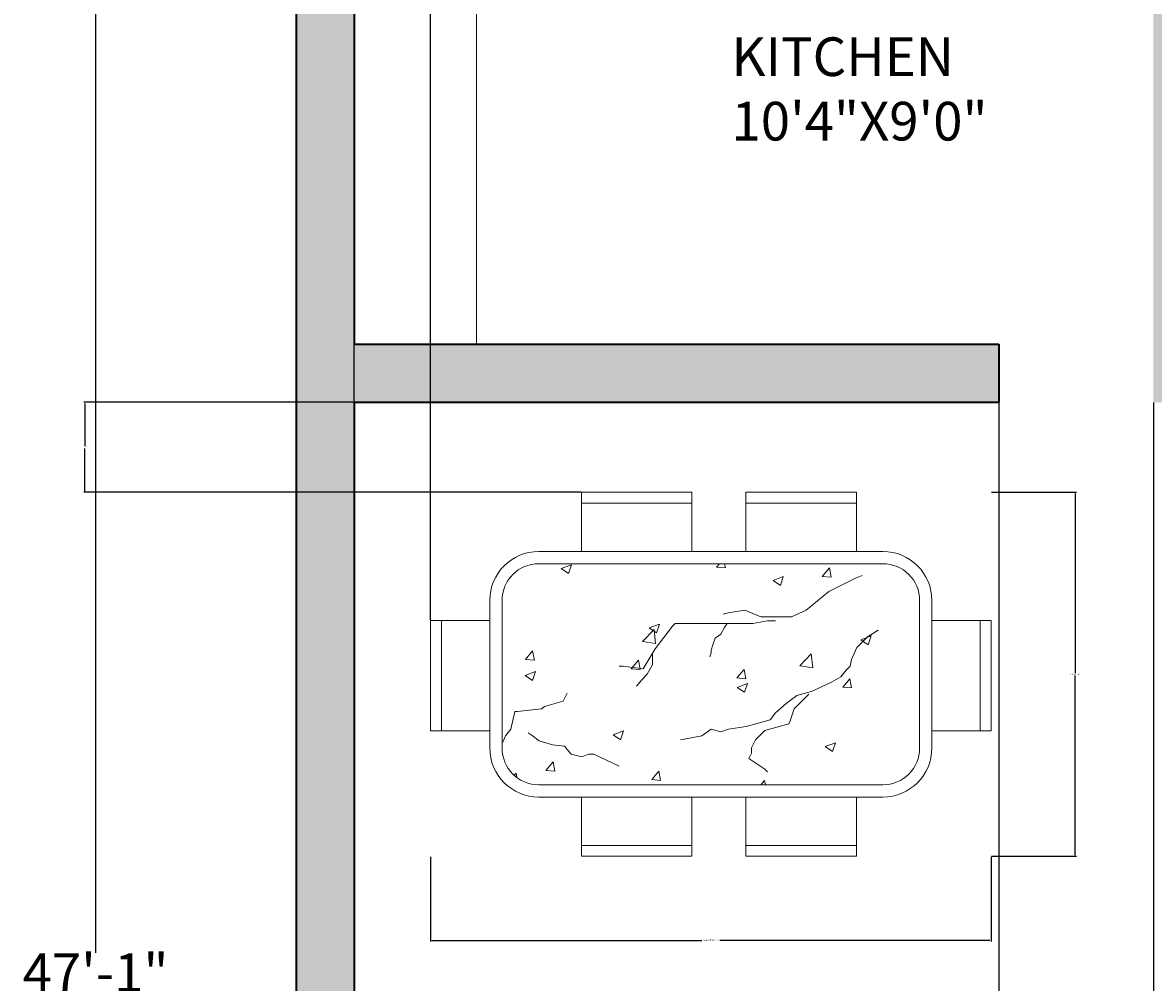
# Model space of a CAD drawing. Units: inches. Extents: x 37 to 706, y -568 to 110.
# Tile 18 of 24: x 37 to 212, y -233 to -84. Entities that reach past the tile are written whole.
import ezdxf

# ---------------------------------------------------------------- set-up
doc = ezdxf.new("R2010")
doc.units = ezdxf.units.IN
doc.header["$MEASUREMENT"] = 0
for name, color, linetype, lineweight in [('A-ANNO-DIMS', 2, 'Continuous', 18), ('A-AREA-IDEN', 7, 'Continuous', 18), ('A-FLOR-CASE', 9, 'Continuous', 18), ('A-FURN', 8, 'Continuous', 13), ('A-WALL', 7, 'Continuous', 35), ('A-WALL-PATT', 252, 'Continuous', 13)]:
    doc.layers.add(name, color=color, linetype=linetype, lineweight=lineweight)
doc.styles.get("Standard").update_dxf_attribs({"font": 'arial.ttf'})
doc.dimstyles.get("Standard").update_dxf_attribs({"dimtxt": 0.18, "dimasz": 0.18, "dimexe": 0.18, "dimexo": 0.0625, "dimgap": 0.09, "dimtad": 0, "dimtih": 1, "dimtoh": 1, "dimdec": 0, "dimzin": 0, "dimdsep": 46, "dimlunit": 3, "dimtxsty": 'Standard', "dimcen": 0.09, "dimadec": 0, "dimazin": 0, "dimtfac": 1, "dimtdec": 0, "dimtofl": 0, "dimtmove": 0, "dimatfit": 3, "dimfxl": 1, "dimtolj": 1, "dimtzin": 0, "dimarcsym": 0})

# ---------------------------------------------------------------- blocks, each defined once
blk = doc.blocks.new('*D3')
at = {"layer": 'A-ANNO-DIMS', "color": 0, "lineweight": -2, "transparency": 16777216}
for p, q in [((78.9, 51.29), (47.67, 51.29)), ((47.85, 51.11), (47.85, -228.11)), ((47.85, -513.53), (47.85, -234.31)), ((78.9, -513.71), (47.67, -513.71))]:
    blk.add_line(p, q, dxfattribs=at)
at = {"layer": 'A-ANNO-DIMS', "color": 0, "transparency": 16777216}
for points in [[(47.82, 51.11), (47.88, 51.11), (47.85, 51.29)], [(47.82, -513.53), (47.88, -513.53), (47.85, -513.71)]]:
    blk.add_solid(points, dxfattribs=at)
at = {"layer": 'Defpoints', "color": 0, "transparency": 16777216}
for p in [(78.96, 51.29), (47.85, -513.71), (78.96, -513.71)]:
    blk.add_point(p, dxfattribs=at)
at = {"layer": 'A-ANNO-DIMS', "color": 0, "transparency": 16777216, "insert": (47.85, -231.21), "char_height": 6, "attachment_point": 5}
blk.add_mtext('\\A1;47\'-1"', dxfattribs=at)
blk = doc.blocks.new('DINING-SET-6')
for p, q in [((23.4, 47.29), (23.4, 56.48)), ((23.4, 56.48), (40.55, 56.48)), ((40.55, 56.48), (40.55, 47.29)), ((48.93, 47.29), (48.93, 56.48)), ((48.93, 56.48), (66.08, 56.48)), ((66.08, 56.48), (66.08, 47.29)), ((40.55, 54.8), (23.4, 54.8)), ((66.08, 54.8), (48.93, 54.8)), ((70.16, 47.29), (16.81, 47.29)), ((16.81, 45.39), (70.16, 45.39)), ((20.27, 44.63), (21.87, 45.24)), ((20.27, 44.63), (21.41, 43.86)), ((21.41, 43.86), (21.87, 45.24)), ((44.37, 44.86), (44.81, 45.39)), ((44.37, 44.86), (45.74, 44.74)), ((45.74, 44.74), (45.62, 45.39)), ((60.77, 43.43), (61.87, 44.74)), ((62.14, 43.31), (61.87, 44.74)), ((53.13, 42.8), (54.73, 43.41)), ((53.13, 42.8), (54.27, 42.03)), ((54.27, 42.03), (54.73, 43.41)), ((60.77, 43.43), (62.14, 43.31)), ((65.93, 43.13), (61.79, 41.06)), ((66.97, 43.54), (65.93, 43.13)), ((61.79, 41.06), (58.27, 38.16)), ((9.18, 39.67), (9.18, 16.81)), ((11.09, 16.81), (11.09, 39.67)), ((75.87, 39.67), (75.87, 16.81)), ((77.78, 16.81), (77.78, 39.67)), ((46.25, 37.75), (45.42, 37.54)), ((48.74, 38.16), (46.25, 37.75)), ((51.22, 37.13), (48.74, 38.16)), ((55.99, 37.13), (51.22, 37.13)), ((58.27, 38.16), (55.99, 37.13)), ((0, 36.58), (0, 19.44)), ((9.18, 36.58), (0, 36.58)), ((1.68, 19.44), (1.68, 36.58)), ((32.89, 33.34), (34.67, 35.2)), ((33.92, 35.42), (35.52, 36.03)), ((33.92, 35.42), (35.05, 34.65)), ((34.92, 33.03), (34.67, 35.2)), ((37.55, 35.68), (34.85, 32.16)), ((35.05, 34.65), (35.52, 36.03)), ((37.96, 36.09), (37.55, 35.68)), ((49.98, 36.09), (37.96, 36.09)), ((45.63, 35.48), (45.01, 34.45)), ((46.04, 36.1), (45.63, 35.48)), ((52.26, 36.51), (49.98, 36.09)), ((53.5, 36.51), (52.26, 36.51)), ((86.96, 36.58), (77.78, 36.58)), ((85.29, 36.58), (85.29, 19.44)), ((86.96, 19.44), (86.96, 36.58)), ((32.89, 33.34), (34.92, 33.03)), ((44.18, 33.82), (43.77, 32.79)), ((45.01, 34.45), (44.18, 33.82)), ((67.8, 34.02), (66.14, 32.37)), ((66.78, 33.59), (68.38, 34.2)), ((66.78, 33.59), (67.91, 32.82)), ((69.45, 35.06), (67.8, 34.02)), ((67.91, 32.82), (68.38, 34.2)), ((14.74, 30.53), (15.84, 31.85)), ((16.11, 30.41), (15.84, 31.85)), ((34.85, 32.16), (32.99, 29.06)), ((43.77, 32.79), (43.56, 31.96)), ((43.56, 31.96), (43.56, 31.55)), ((66.14, 32.37), (65.31, 30.51)), ((14.74, 30.53), (16.11, 30.41)), ((31.14, 29.1), (32.24, 30.41)), ((32.51, 28.98), (32.24, 30.41)), ((34.44, 31.54), (34.44, 29.68)), ((43.56, 31.55), (43.35, 30.93)), ((57.29, 29.56), (59.07, 31.41)), ((59.33, 29.24), (59.07, 31.41)), ((65.31, 30.51), (65.1, 29.47)), ((14.7, 28.05), (16.31, 28.66)), ((15.84, 27.28), (16.31, 28.66)), ((29.88, 29.47), (29.26, 29.47)), ((32.99, 29.06), (29.88, 29.47)), ((31.14, 29.1), (32.51, 28.98)), ((33.61, 28.23), (32.78, 27.4)), ((34.44, 29.68), (33.61, 28.23)), ((47.54, 27.66), (48.64, 28.98)), ((48.91, 27.54), (48.65, 28.98)), ((57.29, 29.56), (59.32, 29.24)), ((64.48, 28.85), (63.65, 27.82)), ((65.1, 29.47), (64.48, 28.85)), ((14.7, 28.05), (15.84, 27.28)), ((32.78, 27.4), (31.95, 26.37)), ((47.54, 27.66), (48.91, 27.54)), ((47.56, 26.21), (49.17, 26.83)), ((48.7, 25.45), (49.17, 26.83)), ((62.2, 26.99), (59.09, 25.54)), ((63.65, 27.82), (62.2, 26.99)), ((63.94, 26.23), (65.05, 27.54)), ((65.31, 26.11), (65.05, 27.54)), ((20.56, 24.09), (21.18, 25.33)), ((47.56, 26.21), (48.7, 25.45)), ((56.82, 24.92), (55.16, 23.68)), ((59.09, 25.54), (56.82, 24.92)), ((58.68, 25.13), (57.85, 24.3)), ((63.94, 26.23), (65.31, 26.11)), ((13.51, 22.44), (17.24, 22.85)), ((17.24, 22.85), (17.66, 23.26)), ((17.66, 23.26), (20.56, 24.09)), ((55.16, 23.68), (53.5, 22.23)), ((56.4, 22.85), (55.78, 20.99)), ((57.85, 24.3), (56.4, 22.85)), ((12.48, 19.74), (13.1, 22.44)), ((13.1, 22.44), (13.51, 22.44)), ((52.67, 21.19), (48.94, 20.16)), ((53.5, 22.23), (52.67, 21.19)), ((0, 19.44), (9.18, 19.44)), ((11.65, 18.71), (12.48, 19.74)), ((28.35, 18.84), (29.95, 19.45)), ((29.49, 18.07), (29.95, 19.45)), ((43.56, 19.74), (42.11, 18.71)), ((45.01, 19.33), (43.56, 19.74)), ((46.25, 19.74), (45.01, 19.33)), ((48.94, 20.16), (46.25, 19.74)), ((51.84, 19.54), (50.39, 18.09)), ((55.57, 20.57), (51.84, 19.54)), ((55.78, 20.99), (55.57, 20.57)), ((77.78, 19.44), (86.96, 19.44)), ((11.23, 17.68), (11.65, 18.71)), ((15.79, 18.72), (15.17, 19.13)), ((16.83, 17.89), (15.79, 18.72)), ((18.9, 17.27), (16.83, 17.89)), ((28.35, 18.84), (29.49, 18.07)), ((42.11, 18.71), (38.79, 18.09)), ((50.39, 18.09), (49.77, 16.85)), ((61.21, 17.01), (62.81, 17.62)), ((62.35, 16.24), (62.81, 17.62)), ((20.77, 17.06), (18.9, 17.27)), ((21.8, 15.82), (20.77, 17.06)), ((23.46, 15.41), (21.8, 15.82)), ((24.5, 15.82), (23.46, 15.41)), ((25.33, 15.82), (24.5, 15.82)), ((29.26, 13.96), (25.33, 15.82)), ((49.77, 16.02), (49.36, 15.19)), ((49.77, 16.85), (49.77, 16.02)), ((61.21, 17.01), (62.35, 16.24)), ((17.91, 13.33), (19.02, 14.65)), ((19.28, 13.21), (19.02, 14.65)), ((49.36, 15.19), (51.84, 13.54)), ((12.96, 12.57), (13.3, 12.92)), ((13.38, 12.23), (13.3, 12.92)), ((17.91, 13.33), (19.28, 13.22)), ((34.31, 11.9), (35.42, 13.21)), ((35.68, 11.78), (35.42, 13.21)), ((51.84, 13.54), (52.26, 13.12)), ((70.16, 11.09), (16.81, 11.09)), ((34.31, 11.9), (35.68, 11.78)), ((51.24, 11.09), (51.82, 11.78)), ((51.94, 11.09), (51.82, 11.78)), ((16.81, 9.18), (70.16, 9.18)), ((23.4, 9.18), (23.4, 0)), ((40.55, 0), (40.55, 9.18)), ((48.93, 9.18), (48.93, 0)), ((66.08, 0), (66.08, 9.18)), ((40.55, 1.68), (23.4, 1.68)), ((23.4, 0), (40.55, 0)), ((66.08, 1.68), (48.93, 1.68)), ((48.93, 0), (66.08, 0))]:
    blk.add_line(p, q)
for centre, radius, start, end in [((16.81, 39.67), 7.62, 90, 180), ((70.16, 39.67), 7.62, 0, 90), ((16.81, 39.67), 5.72, 90, 180), ((70.16, 39.67), 5.72, 0, 90), ((16.81, 16.81), 7.62, 180, 270), ((16.81, 16.81), 5.72, 180, 270), ((70.16, 16.81), 5.72, 270, 0), ((70.16, 16.81), 7.62, 270, 0)]:
    blk.add_arc(centre, radius, start, end)
blk = doc.blocks.new('*D31')
at = {"layer": 'A-ANNO-DIMS', "color": 0, "lineweight": -2, "transparency": 16777216}
for p, q in [((99.82, -213.21), (99.82, -226.37)), ((186.78, -213.21), (186.78, -226.37)), ((100, -226.19), (141.91, -226.19)), ((186.6, -226.19), (144.69, -226.19))]:
    blk.add_line(p, q, dxfattribs=at)
at = {"layer": 'A-ANNO-DIMS', "color": 0, "transparency": 16777216}
for points in [[(100, -226.16), (100, -226.22), (99.82, -226.19)], [(186.6, -226.16), (186.6, -226.22), (186.78, -226.19)]]:
    blk.add_solid(points, dxfattribs=at)
at = {"layer": 'Defpoints', "color": 0, "transparency": 16777216}
for p in [(99.82, -213.15), (186.78, -213.15), (186.78, -226.19)]:
    blk.add_point(p, dxfattribs=at)
at = {"layer": 'A-ANNO-DIMS', "color": 0, "transparency": 16777216, "insert": (143.3, -226.19), "char_height": 0.18, "attachment_point": 5}
blk.add_mtext('\\A1;DINING SET 7\'-3" TYP.', dxfattribs=at)
blk = doc.blocks.new('*D32')
at = {"layer": 'A-ANNO-DIMS', "color": 0, "lineweight": -2, "transparency": 16777216}
for p, q in [((186.84, -156.67), (200.01, -156.67)), ((199.83, -156.85), (199.83, -184.73)), ((199.83, -212.97), (199.83, -185.09)), ((186.84, -213.15), (200.01, -213.15))]:
    blk.add_line(p, q, dxfattribs=at)
at = {"layer": 'A-ANNO-DIMS', "color": 0, "transparency": 16777216}
for points in [[(199.8, -156.85), (199.86, -156.85), (199.83, -156.67)], [(199.8, -212.97), (199.86, -212.97), (199.83, -213.15)]]:
    blk.add_solid(points, dxfattribs=at)
at = {"layer": 'Defpoints', "color": 0, "transparency": 16777216}
for p in [(186.78, -156.67), (199.83, -156.67), (186.78, -213.15)]:
    blk.add_point(p, dxfattribs=at)
at = {"layer": 'A-ANNO-DIMS', "color": 0, "transparency": 16777216, "insert": (199.83, -184.91), "char_height": 0.18, "attachment_point": 5}
blk.add_mtext('\\A1;4\'-8 1/2" TYP.', dxfattribs=at)
blk = doc.blocks.new('*D60')
at = {"layer": 'A-ANNO-DIMS', "color": 0, "lineweight": -2, "transparency": 16777216}
for p, q in [((87.96, -142.65), (87.96, 84.22)), ((99.82, -176.5), (99.82, 84.22)), ((88.14, 84.04), (93.57, 84.04)), ((99.64, 84.04), (94.21, 84.04))]:
    blk.add_line(p, q, dxfattribs=at)
at = {"layer": 'A-ANNO-DIMS', "color": 0, "transparency": 16777216}
for points in [[(88.14, 84.07), (88.14, 84.01), (87.96, 84.04)], [(99.64, 84.07), (99.64, 84.01), (99.82, 84.04)]]:
    blk.add_solid(points, dxfattribs=at)
at = {"layer": 'Defpoints', "color": 0, "transparency": 16777216}
for p in [(99.82, 84.04), (87.96, -142.71), (99.82, -176.56)]:
    blk.add_point(p, dxfattribs=at)
at = {"layer": 'A-ANNO-DIMS', "color": 0, "transparency": 16777216, "insert": (93.89, 84.04), "char_height": 0.18, "attachment_point": 5}
blk.add_mtext('\\A1;1\'-0"', dxfattribs=at)
blk = doc.blocks.new('*D61')
at = {"layer": 'A-ANNO-DIMS', "color": 0, "lineweight": -2, "transparency": 16777216}
for p, q in [((87.9, -142.71), (46.03, -142.71)), ((46.21, -142.89), (46.21, -149.51)), ((46.21, -156.49), (46.21, -149.87)), ((123.15, -156.67), (46.03, -156.67))]:
    blk.add_line(p, q, dxfattribs=at)
at = {"layer": 'A-ANNO-DIMS', "color": 0, "transparency": 16777216}
for points in [[(46.18, -142.89), (46.24, -142.89), (46.21, -142.71)], [(46.18, -156.49), (46.24, -156.49), (46.21, -156.67)]]:
    blk.add_solid(points, dxfattribs=at)
at = {"layer": 'Defpoints', "color": 0, "transparency": 16777216}
for p in [(87.96, -142.71), (46.21, -156.67), (123.22, -156.67)]:
    blk.add_point(p, dxfattribs=at)
at = {"layer": 'A-ANNO-DIMS', "color": 0, "transparency": 16777216, "insert": (46.21, -149.69), "char_height": 0.18, "attachment_point": 5}
blk.add_mtext('\\A1;1\'-2"', dxfattribs=at)
blk = doc.blocks.new('*D62')
at = {"layer": 'A-ANNO-DIMS', "color": 0, "lineweight": -2, "transparency": 16777216}
for p, q in [((187.96, -142.77), (187.96, -567.64)), ((211.96, -142.77), (211.96, -567.64)), ((188.14, -567.46), (199.63, -567.46)), ((211.78, -567.46), (200.29, -567.46))]:
    blk.add_line(p, q, dxfattribs=at)
at = {"layer": 'A-ANNO-DIMS', "color": 0, "transparency": 16777216}
for points in [[(188.14, -567.43), (188.14, -567.49), (187.96, -567.46)], [(211.78, -567.43), (211.78, -567.49), (211.96, -567.46)]]:
    blk.add_solid(points, dxfattribs=at)
at = {"layer": 'Defpoints', "color": 0, "transparency": 16777216}
for p in [(187.96, -142.71), (211.96, -142.71), (211.96, -567.46)]:
    blk.add_point(p, dxfattribs=at)
at = {"layer": 'A-ANNO-DIMS', "color": 0, "transparency": 16777216, "insert": (199.96, -567.46), "char_height": 0.18, "attachment_point": 5}
blk.add_mtext('\\A1;2\'-0"', dxfattribs=at)

msp = doc.modelspace()

# ---------------------------------------------------------------- hatches: boundary and pattern name
at = {"layer": 'A-WALL-PATT'}
h = msp.add_hatch(color=256, dxfattribs=at)
h.dxf.hatch_style = 1
h.paths.add_polyline_path([(220.96, -351.71), (211.96, -351.71), (211.96, -513.71), (254.96, -513.71), (254.96, -504.71), (220.96, -504.71)], flags=17)
h.paths.add_polyline_path([(220.96, -294.71), (211.96, -294.71), (211.96, -303.71), (220.96, -303.71)], flags=17)
h.paths.add_polyline_path([(175.96, -294.71), (155.87, -294.71), (155.87, -303.71), (155.96, -303.71), (175.96, -303.71)], flags=17)
h.paths.add_polyline_path([(220.96, -16.71), (211.96, -16.71), (211.96, -142.71), (220.96, -142.71)], flags=17)
h.paths.add_polyline_path([(357.96, 51.29), (78.96, 51.29), (78.96, -513.71), (87.96, -513.71), (87.96, -303.71), (95.87, -303.71), (95.87, -294.71), (87.96, -294.71), (87.96, -142.71), (187.96, -142.71), (187.96, -133.71), (87.96, -133.71), (87.96, -25.71), (106.96, -25.71), (106.96, -16.71), (87.96, -16.71), (87.96, 42.29), (348.96, 42.29), (348.96, 17.13), (348.96, -133.71), (246.96, -133.71), (246.96, -142.71), (348.96, -142.71), (348.96, -294.71), (251.96, -294.71), (251.96, -303.71), (348.96, -303.71), (348.96, -351.71), (260.96, -351.71), (260.96, -329.71), (251.96, -329.71), (251.96, -360.71), (327.45, -360.71), (348.96, -360.71), (348.96, -504.71), (314.96, -504.71), (314.96, -513.71), (357.96, -513.71)])
h.paths.add_polyline_path([(416.96, -303.71), (402.96, -303.71), (402.96, -151.71), (478.96, -151.71), (478.96, -142.71), (402.96, -142.71), (402.96, -22.71), (409.96, -22.71), (409.96, -13.71), (402.96, -13.71), (402.96, 42.29), (663.96, 42.29), (663.96, -303.71), (566.96, -303.71), (566.96, -312.71), (663.96, -312.71), (663.96, -360.71), (575.96, -360.71), (575.96, -338.71), (566.96, -338.71), (566.96, -360.71), (566.96, -369.71), (642.45, -369.71), (663.96, -369.71), (663.96, -513.71), (629.96, -513.71), (629.96, -522.71), (672.96, -522.71), (672.96, 51.29), (393.96, 51.29), (393.96, -522.71), (402.96, -522.71), (402.96, -312.71), (416.96, -312.71)])
h.paths.add_polyline_path([(490.96, -303.71), (476.96, -303.71), (476.96, -312.71), (490.96, -312.71)], flags=17)
h.paths.add_polyline_path([(535.96, -303.71), (526.96, -303.71), (526.96, -312.71), (535.96, -312.71)], flags=17)
h.paths.add_polyline_path([(535.96, -369.71), (526.96, -369.71), (526.96, -522.71), (569.96, -522.71), (569.96, -513.71), (535.96, -513.71)], flags=17)
h.paths.add_polyline_path([(511.96, -13.71), (502.96, -13.71), (502.96, -151.71), (511.96, -151.71)], flags=17)
h.paths.add_polyline_path([(651.54, -142.71), (651.54, -120.18), (642.54, -120.18), (642.54, -142.71), (550.54, -142.71), (550.54, -120.71), (541.54, -120.71), (541.54, -142.71), (537.96, -142.71), (537.96, -151.71), (651.54, -151.71)], flags=17)
h.paths.add_polyline_path([(651.54, -85.71), (541.54, -85.71), (541.54, -94.71), (651.54, -94.71)], flags=17)
h.paths.add_polyline_path([(476.96, -13.71), (469.96, -13.71), (469.96, -22.71), (476.96, -22.71)], flags=17)
h.paths.add_polyline_path([(185.96, -16.71), (166.96, -16.71), (166.96, -25.71), (185.96, -25.71)], flags=17)
h.paths.add_polyline_path([(168.91, -414.72), (214.62, -414.72), (214.62, -392.33), (168.91, -392.33)], flags=25)

# ---------------------------------------------------------------- linework, layer by layer
at = {"layer": 'A-FLOR-CASE'}
msp.add_line((106.97, -46.61), (106.97, -133.71), dxfattribs=at)
at = {"layer": 'A-WALL'}
for p, q in [((78.96, 51.29), (78.96, -513.71)), ((87.96, -25.71), (87.96, -133.71)), ((87.96, -133.71), (187.96, -133.71)), ((187.96, -133.71), (187.96, -142.71)), ((87.96, -142.71), (187.96, -142.71)), ((87.96, -142.71), (87.96, -294.71))]:
    msp.add_line(p, q, dxfattribs=at)

# ---------------------------------------------------------------- block references
at = {"layer": 'A-FURN'}
msp.add_blockref('DINING-SET-6', (99.82, -213.15), dxfattribs=at)

# ---------------------------------------------------------------- texts
at = {"layer": 'A-AREA-IDEN', "insert": (146.51, -86.11), "char_height": 6, "attachment_point": 1}
msp.add_mtext('KITCHEN\\P10\'4"X9\'0"', dxfattribs=at)

# ---------------------------------------------------------------- dimensions: what is measured, and where the dimension line sits
at = {"layer": 'A-ANNO-DIMS'}
for base, p1, p2, picture, middle in [((99.82, 84.04), (87.96, -142.71), (99.82, -176.56), '*D60', (93.89, 84.04)), ((211.96, -567.46), (187.96, -142.71), (211.96, -142.71), '*D62', (199.96, -567.46))]:
    dim = msp.add_linear_dim(base=base, p1=p1, p2=p2, dimstyle='Standard', override={"dimdec": 1, "dimlfac": 1, "dimrnd": 0, "dimzin": 1, "dimdsep": 46, "dimlunit": 4, "dimfrac": 2}, dxfattribs=at)
    dim.commit()
    dim.dimension.update_dxf_attribs({"geometry": picture, "text_midpoint": middle})
for base, p1, p2, override, picture, middle in [((47.85, -513.71), (78.96, 51.29), (78.96, -513.71), {"dimtxt": 6, "dimclrd": 0, "dimclre": 0, "dimclrt": 0}, '*D3', (47.85, -231.21)), ((46.21, -156.67), (87.96, -142.71), (123.22, -156.67), {"dimdec": 1, "dimlfac": 1, "dimrnd": 0, "dimzin": 1, "dimdsep": 46, "dimlunit": 4, "dimfrac": 2}, '*D61', (46.21, -149.69))]:
    dim = msp.add_linear_dim(base=base, p1=p1, p2=p2, angle=90, dimstyle='Standard', override=override, dxfattribs=at)
    dim.commit()
    dim.dimension.update_dxf_attribs({"geometry": picture, "text_midpoint": middle})
dim = msp.add_linear_dim(base=(199.83, -156.67), p1=(186.78, -213.15), p2=(186.78, -156.67), angle=90, text='<> TYP.', dimstyle='Standard', override={"dimdec": 1, "dimlfac": 1, "dimrnd": 0, "dimzin": 1, "dimdsep": 46, "dimlunit": 4, "dimfrac": 2}, dxfattribs=at)
dim.commit()
dim.dimension.update_dxf_attribs({"geometry": '*D32', "text_midpoint": (199.83, -184.91)})
dim = msp.add_linear_dim(base=(186.78, -226.19), p1=(99.82, -213.15), p2=(186.78, -213.15), text='DINING SET <> TYP.', dimstyle='Standard', override={"dimdec": 1, "dimlfac": 1, "dimrnd": 0, "dimzin": 1, "dimdsep": 46, "dimlunit": 4, "dimfrac": 2}, dxfattribs=at)
dim.commit()
dim.dimension.update_dxf_attribs({"geometry": '*D31', "text_midpoint": (143.3, -226.19)})

doc.saveas('drawing.dxf')
